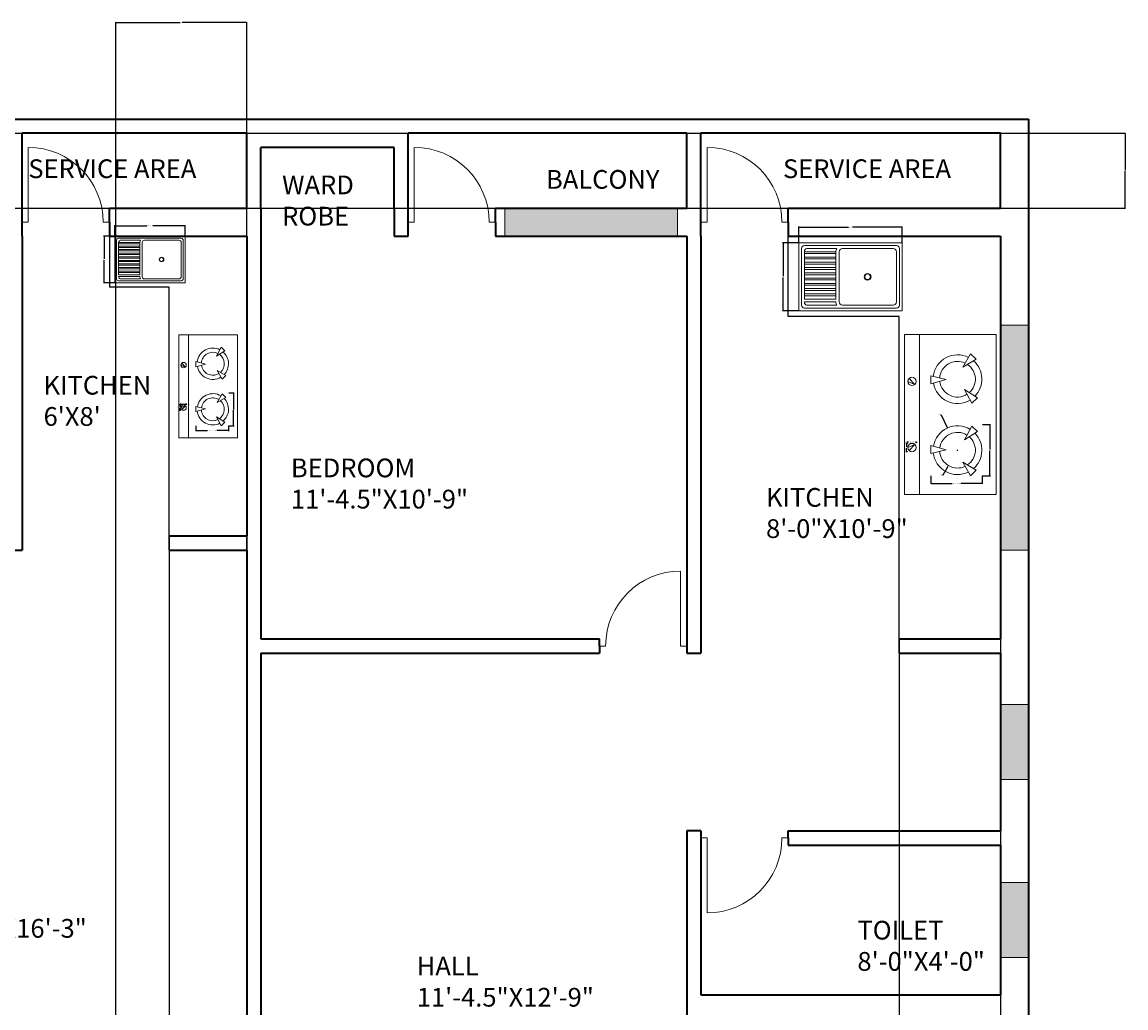
# Model space of a CAD drawing. Units: inches. Extents: x -89 to 565, y -517 to 71.
# Tile 3 of 3: x 211 to 565, y -245 to 71. Entities that reach past the tile are written whole.
import ezdxf

# ---------------------------------------------------------------- set-up
doc = ezdxf.new("R2010")
doc.units = ezdxf.units.IN
doc.header["$MEASUREMENT"] = 0
for name, color, linetype, lineweight in [('A-ANNO-DIMS', 2, 'Continuous', 18), ('A-AREA-IDEN', 7, 'Continuous', 18), ('A-DOOR', 4, 'Continuous', 18), ('A-EQPM', 8, 'Continuous', 18), ('A-FLOR-CASE', 8, 'Continuous', 25), ('A-FLOR-FIXT', 8, 'Continuous', 18), ('A-GLAZ', 3, 'Continuous', 18), ('A-GLAZ-PATT', 9, 'Continuous', 13), ('A-WALL', 7, 'Continuous', 35)]:
    doc.layers.add(name, color=color, linetype=linetype, lineweight=lineweight)
doc.styles.get("Standard").update_dxf_attribs({"font": 'arial.ttf'})
doc.dimstyles.get("Standard").update_dxf_attribs({"dimtxt": 0.18, "dimasz": 0.18, "dimexe": 0.18, "dimexo": 0.0625, "dimgap": 0.09, "dimtad": 0, "dimtih": 1, "dimtoh": 1, "dimdec": 0, "dimzin": 0, "dimdsep": 46, "dimlunit": 3, "dimtxsty": 'Standard', "dimcen": 0.09, "dimadec": 0, "dimazin": 0, "dimtfac": 1, "dimtdec": 0, "dimtofl": 0, "dimtmove": 0, "dimatfit": 3, "dimfxl": 1, "dimtolj": 1, "dimtzin": 0, "dimarcsym": 0})

# ---------------------------------------------------------------- blocks, each defined once
blk = doc.blocks.new('М12 540х820')
for p, q in [((0, 540), (-820, 540)), ((-820, 540), (-820, 0)), ((0, 0), (0, 540)), ((-797.5, 495), (-797.5, 45)), ((-45, 517.5), (-775, 517.5)), ((-775, 468), (-775, 72)), ((-347.5, 495), (-748, 495)), ((-320.5, 468), (-320.5, 72)), ((-301.7, 495), (-64.8, 495)), ((-293.7, 468), (-293.7, 472.5)), ((-293.7, 468), (-45, 468)), ((-293.7, 446.6), (-45, 446.6)), ((-293.7, 419.6), (-293.7, 446.6)), ((-45, 469.5), (-45, 468)), ((-45, 419.6), (-45, 446.6)), ((-22.5, 45), (-22.5, 495)), ((-293.7, 419.6), (-45, 419.6)), ((-293.7, 405), (-45, 405)), ((-293.7, 378), (-293.7, 405)), ((-293.7, 378), (-45, 378)), ((-293.7, 336.4), (-293.7, 363.4)), ((-293.7, 363.4), (-45, 363.4)), ((-45, 378), (-45, 405)), ((-45, 336.4), (-45, 363.4)), ((-293.7, 336.4), (-45, 336.4)), ((-293.7, 294.7), (-293.7, 321.7)), ((-293.7, 321.7), (-45, 321.7)), ((-293.7, 294.7), (-45, 294.7)), ((-293.7, 253.1), (-293.7, 280.1)), ((-293.7, 280.1), (-45, 280.1)), ((-45, 294.7), (-45, 321.7)), ((-45, 253.1), (-45, 280.1)), ((-293.7, 253.1), (-45, 253.1)), ((-293.7, 211.5), (-293.7, 238.5)), ((-293.7, 238.5), (-45, 238.5)), ((-293.7, 211.5), (-45, 211.5)), ((-293.7, 169.9), (-293.7, 196.9)), ((-293.7, 196.9), (-45, 196.9)), ((-45, 211.5), (-45, 238.5)), ((-45, 169.9), (-45, 196.9)), ((-293.7, 169.9), (-45, 169.9)), ((-293.7, 128.2), (-293.7, 155.2)), ((-293.7, 155.2), (-45, 155.2)), ((-293.7, 128.2), (-45, 128.2)), ((-293.7, 113.6), (-45, 113.6)), ((-293.7, 86.6), (-293.7, 113.6)), ((-45, 128.2), (-45, 155.2)), ((-45, 86.6), (-45, 113.6)), ((-820, 0), (0, 0)), ((-775, 22.5), (-45, 22.5)), ((-748, 45), (-347.5, 45)), ((-301.7, 45), (-64.8, 45)), ((-293.7, 86.6), (-45, 86.6)), ((-293.7, 72), (-45, 72)), ((-45, 70.5), (-45, 72))]:
    blk.add_line(p, q)
at = {"ltscale": 0.06}
for p, q in [((-820, 0), (-820, 540)), ((-820, 540), (0, 540)), ((0, 540), (0, 536.9)), ((0, 536.9), (0, 0)), ((-293.7, 446.6), (-45, 446.6)), ((-293.7, 405), (-293.7, 446.6)), ((-45, 446.6), (-45, 419.6)), ((-293.7, 363.4), (-293.7, 405)), ((-293.7, 321.7), (-293.7, 363.4)), ((-45, 419.6), (-45, 378)), ((-45, 378), (-45, 336.4)), ((-293.7, 280.1), (-293.7, 321.7)), ((-293.7, 238.5), (-293.7, 280.1)), ((-45, 336.4), (-45, 294.7)), ((-45, 294.7), (-45, 253.1)), ((-293.7, 196.9), (-293.7, 238.5)), ((-293.7, 155.2), (-293.7, 196.9)), ((-45, 253.1), (-45, 211.5)), ((-45, 211.5), (-45, 169.9)), ((-293.7, 113.6), (-293.7, 155.2)), ((-293.7, 72), (-293.7, 113.6)), ((-45, 169.9), (-45, 128.2)), ((-45, 128.2), (-45, 86.6)), ((0, 0), (-820, 0)), ((-45, 72), (-293.7, 72)), ((-45, 86.6), (-45, 72))]:
    blk.add_line(p, q, dxfattribs=at)
at = {"extrusion": (0, 0, -1)}
for centre, major_axis, start_param, end_param in [((-775, 495), (-15.9, 15.9), -0.785398, 0.785398), ((-775, 495), (-15.9, 15.9), -0.785398, 0.785398), ((-748, 468), (-19.1, -19.1), 0.785398, 2.356194), ((-748, 468), (-19.1, -19.1), 0.785398, 2.356194), ((-347.5, 468), (-19.1, 19.1), 0.785398, 2.356194), ((-347.5, 468), (-19.1, 19.1), 0.785398, 2.356194), ((-343.2, 468), (-35, 35), 1.779263, 2.356194), ((-343.2, 468), (-35, 35), 1.779263, 2.356192), ((-343.2, 468), (-35, 35), 2.356192, 2.356194), ((-72.3, 468.8), (-19.3, 19.3), 1.0328, 2.38382), ((-72.3, 468.8), (-19.3, 19.3), 1.0328, 1.064673), ((-72.3, 468.8), (-19.3, 19.3), 1.064673, 2.328569), ((-45, 495), (-15.9, -15.9), 2.356194, 3.926991), ((-45, 495), (-15.9, -15.9), 2.356194, 3.926991), ((-72.3, 468.8), (-19.3, 19.3), 2.328569, 2.38382), ((-545.5, 270), (-19.1, -19.1), 3.926991, 10.210176), ((-545.5, 270), (-19.1, -19.1), 3.926991, 10.210176), ((-545.5, 270), (-15.9, -15.9), 3.926991, 10.210176), ((-545.5, 270), (-15.9, -15.9), 3.926991, 10.210176), ((-775, 45), (-15.9, -15.9), 5.497787, 7.068583), ((-775, 45), (-15.9, -15.9), 5.497787, 7.068583), ((-748, 72), (-19.1, 19.1), 3.926991, 5.497787), ((-748, 72), (-19.1, 19.1), 3.926991, 5.497787), ((-347.5, 72), (-19.1, -19.1), 3.926991, 5.497787), ((-347.5, 72), (-19.1, -19.1), 3.926991, 5.497787), ((-343.2, 72), (-35, -35), 3.926991, 4.503922), ((-343.2, 72), (-35, -35), 3.926991, 4.503922), ((-72.3, 71.2), (-19.3, -19.3), 3.899365, 5.250385), ((-72.3, 71.2), (-19.3, -19.3), 5.218512, 5.250385), ((-72.3, 71.2), (-19.3, -19.3), 3.954617, 5.218512), ((-72.3, 71.2), (-19.3, -19.3), 3.899365, 3.954617), ((-45, 45), (-15.9, 15.9), 2.356194, 3.926991), ((-45, 45), (-15.9, 15.9), 2.356194, 3.926991)]:
    blk.add_ellipse(centre, major_axis=major_axis, ratio=1, start_param=start_param, end_param=end_param, dxfattribs=at)
blk = doc.blocks.new('DOOR-SWING-24IN')
for p, q in [((0, 0), (0, 24)), ((-24, 0), (-26, 0)), ((2, 0), (0, 0))]:
    blk.add_line(p, q)
blk.add_arc((0, 0), 24, 90, 180)
blk = doc.blocks.new('COOKTOP-BURNER-LARGE')
for p, q in [((2.2, 3.33), (4.59, 7.69)), ((4.59, 7.69), (6.45, 5.97)), ((6.45, 5.97), (2.2, 3.33)), ((-8.51, -1.06), (-8.51, 1.48)), ((-8.51, 1.48), (-3.69, 0.15)), ((-3.69, 0.15), (-8.51, -1.06)), ((4.18, -8.17), (1.75, -3.8)), ((1.75, -3.8), (5.99, -6.39)), ((5.99, -6.39), (4.18, -8.17))]:
    blk.add_line(p, q)
for radius, start, end in [(7.81, 58.853, 170.7562), (5.72, 57.9778, 173.02), (5.72, 304.5561, 48.8027), (7.81, 311.2225, 44.1627), (7.81, 186.4005, 296.769), (5.72, 183.5753, 295.9207)]:
    blk.add_arc((0, 0), radius, start, end)
blk = doc.blocks.new('COOKTOP-KNOB-LARGE')
at = {"ltscale": 20}
for p, q in [((-1.35, 0), (0.95, 0.96)), ((0.95, 0.96), (-0.95, -0.96))]:
    blk.add_line(p, q, dxfattribs=at)
blk.add_circle((0, 0), 1.35, dxfattribs=at)
blk = doc.blocks.new('COOKTOP-BURNER-COMPACT')
for p, q in [((1.41, 2.14), (2.95, 4.94)), ((4.14, 3.83), (1.41, 2.14)), ((2.95, 4.94), (4.14, 3.83)), ((-5.47, -0.68), (-5.47, 0.95)), ((-5.47, 0.95), (-2.37, 0.1)), ((-2.37, 0.1), (-5.47, -0.68)), ((2.69, -5.25), (1.13, -2.44)), ((1.13, -2.44), (3.85, -4.11)), ((3.85, -4.11), (2.69, -5.25))]:
    blk.add_line(p, q)
for radius, start, end in [(5.02, 58.853, 170.7562), (3.68, 57.9778, 173.02), (3.68, 304.5561, 48.8027), (5.02, 311.2225, 44.1627), (5.02, 186.4005, 296.769), (3.68, 183.5753, 295.9207)]:
    blk.add_arc((0, 0), radius, start, end)
blk = doc.blocks.new('COOKTOP-KNOB-COMPACT')
at = {"ltscale": 20}
for p, q in [((-0.87, 0), (0.61, 0.61)), ((0.61, 0.61), (-0.61, -0.61))]:
    blk.add_line(p, q, dxfattribs=at)
blk.add_circle((0, 0), 0.866, dxfattribs=at)
blk = doc.blocks.new('*D14')
at = {"layer": 'A-ANNO-DIMS', "color": 0, "lineweight": -2, "transparency": 16777216}
for p, q in [((240.77, 1.98), (240.77, 5.48)), ((240.95, 5.3), (251.12, 5.3)), ((263.17, 5.3), (252.99, 5.3)), ((263.35, 1.98), (263.35, 5.48))]:
    blk.add_line(p, q, dxfattribs=at)
at = {"layer": 'A-ANNO-DIMS', "color": 0, "transparency": 16777216}
for points in [[(240.95, 5.33), (240.95, 5.27), (240.77, 5.3)], [(263.17, 5.33), (263.17, 5.27), (263.35, 5.3)]]:
    blk.add_solid(points, dxfattribs=at)
at = {"layer": 'Defpoints', "color": 0, "transparency": 16777216}
for p in [(240.77, 5.3), (240.77, 1.91), (263.35, 1.91)]:
    blk.add_point(p, dxfattribs=at)
at = {"layer": 'A-ANNO-DIMS', "color": 0, "transparency": 16777216, "insert": (252.06, 5.3), "char_height": 0.18, "attachment_point": 5}
blk.add_mtext('\\A1;SINK 1\'-10 1/2"', dxfattribs=at)
blk = doc.blocks.new('*D15')
at = {"layer": 'A-ANNO-DIMS', "color": 0, "lineweight": -2, "transparency": 16777216}
for p, q in [((240.71, 1.91), (237.2, 1.91)), ((237.38, 1.73), (237.38, -5.34)), ((237.38, -12.77), (237.38, -5.7)), ((240.71, -12.95), (237.2, -12.95))]:
    blk.add_line(p, q, dxfattribs=at)
at = {"layer": 'A-ANNO-DIMS', "color": 0, "transparency": 16777216}
for points in [[(237.35, 1.73), (237.41, 1.73), (237.38, 1.91)], [(237.35, -12.77), (237.41, -12.77), (237.38, -12.95)]]:
    blk.add_solid(points, dxfattribs=at)
at = {"layer": 'Defpoints', "color": 0, "transparency": 16777216}
for p in [(240.77, 1.91), (237.38, -12.95), (240.77, -12.95)]:
    blk.add_point(p, dxfattribs=at)
at = {"layer": 'A-ANNO-DIMS', "color": 0, "transparency": 16777216, "insert": (237.38, -5.52), "char_height": 0.18, "attachment_point": 5}
blk.add_mtext('\\A1;1\'-3"', dxfattribs=at)
blk = doc.blocks.new('*D16')
at = {"layer": 'A-ANNO-DIMS', "color": 0, "lineweight": -2, "transparency": 16777216}
for p, q in [((459.97, -0.08), (459.97, 5.01)), ((460.15, 4.83), (475.9, 4.83)), ((492.96, 4.83), (477.21, 4.83)), ((493.14, -0.08), (493.14, 5.01))]:
    blk.add_line(p, q, dxfattribs=at)
at = {"layer": 'A-ANNO-DIMS', "color": 0, "transparency": 16777216}
for points in [[(460.15, 4.86), (460.15, 4.8), (459.97, 4.83)], [(492.96, 4.86), (492.96, 4.8), (493.14, 4.83)]]:
    blk.add_solid(points, dxfattribs=at)
at = {"layer": 'Defpoints', "color": 0, "transparency": 16777216}
for p in [(459.97, 4.83), (459.97, -0.14), (493.14, -0.14)]:
    blk.add_point(p, dxfattribs=at)
at = {"layer": 'A-ANNO-DIMS', "color": 0, "transparency": 16777216, "insert": (476.56, 4.83), "char_height": 0.18, "attachment_point": 5}
blk.add_mtext('\\A1;SINK 2\'-9"', dxfattribs=at)
blk = doc.blocks.new('*D17')
at = {"layer": 'A-ANNO-DIMS', "color": 0, "lineweight": -2, "transparency": 16777216}
for p, q in [((459.9, -0.14), (454.81, -0.14)), ((454.99, -0.32), (454.99, -10.89)), ((454.99, -21.81), (454.99, -11.25)), ((459.9, -21.99), (454.81, -21.99))]:
    blk.add_line(p, q, dxfattribs=at)
at = {"layer": 'A-ANNO-DIMS', "color": 0, "transparency": 16777216}
for points in [[(454.96, -0.32), (455.02, -0.32), (454.99, -0.14)], [(454.96, -21.81), (455.02, -21.81), (454.99, -21.99)]]:
    blk.add_solid(points, dxfattribs=at)
at = {"layer": 'Defpoints', "color": 0, "transparency": 16777216}
for p in [(459.97, -0.14), (454.99, -21.99), (459.97, -21.99)]:
    blk.add_point(p, dxfattribs=at)
at = {"layer": 'A-ANNO-DIMS', "color": 0, "transparency": 16777216, "insert": (454.99, -11.07), "char_height": 0.18, "attachment_point": 5}
blk.add_mtext('\\A1;1\'-10"', dxfattribs=at)
blk = doc.blocks.new('*D18')
at = {"layer": 'A-ANNO-DIMS', "color": 0, "lineweight": -2, "transparency": 16777216}
for p, q in [((502.34, -74.83), (502.34, -77.41)), ((502.52, -77.23), (509.13, -77.23)), ((518.56, -77.23), (511.95, -77.23)), ((518.74, -74.83), (518.74, -77.41))]:
    blk.add_line(p, q, dxfattribs=at)
at = {"layer": 'A-ANNO-DIMS', "color": 0, "transparency": 16777216}
for points in [[(502.52, -77.2), (502.52, -77.26), (502.34, -77.23)], [(518.56, -77.2), (518.56, -77.26), (518.74, -77.23)]]:
    blk.add_solid(points, dxfattribs=at)
at = {"layer": 'Defpoints', "color": 0, "transparency": 16777216}
for p in [(502.34, -74.77), (518.74, -74.77), (518.74, -77.23)]:
    blk.add_point(p, dxfattribs=at)
at = {"layer": 'A-ANNO-DIMS', "color": 0, "transparency": 16777216, "insert": (510.54, -77.23), "char_height": 0.18, "attachment_point": 5}
blk.add_mtext('\\A1;BURNER 1\'-4 1/2" TYP.', dxfattribs=at)
blk = doc.blocks.new('*D19')
at = {"layer": 'A-ANNO-DIMS', "color": 0, "lineweight": -2, "transparency": 16777216}
for p, q in [((518.81, -58.42), (521.38, -58.42)), ((521.2, -58.6), (521.2, -66.41)), ((521.2, -74.59), (521.2, -66.78)), ((518.81, -74.77), (521.38, -74.77))]:
    blk.add_line(p, q, dxfattribs=at)
at = {"layer": 'A-ANNO-DIMS', "color": 0, "transparency": 16777216}
for points in [[(521.17, -58.6), (521.23, -58.6), (521.2, -58.42)], [(521.17, -74.59), (521.23, -74.59), (521.2, -74.77)]]:
    blk.add_solid(points, dxfattribs=at)
at = {"layer": 'Defpoints', "color": 0, "transparency": 16777216}
for p in [(518.74, -58.42), (521.2, -58.42), (518.74, -74.77)]:
    blk.add_point(p, dxfattribs=at)
at = {"layer": 'A-ANNO-DIMS', "color": 0, "transparency": 16777216, "insert": (521.2, -66.6), "char_height": 0.18, "attachment_point": 5}
blk.add_mtext('\\A1;1\'-4 1/2" TYP.', dxfattribs=at)
blk = doc.blocks.new('*D20')
at = {"layer": 'A-ANNO-DIMS', "color": 0, "lineweight": -2, "transparency": 16777216}
for p, q in [((494.74, -64.01), (494.56, -64.01)), ((494.92, -64.35), (494.92, -63.83)), ((497.61, -64.35), (497.61, -63.83)), ((497.79, -64.01), (497.97, -64.01))]:
    blk.add_line(p, q, dxfattribs=at)
at = {"layer": 'A-ANNO-DIMS', "color": 0, "transparency": 16777216}
for points in [[(494.74, -63.98), (494.74, -64.04), (494.92, -64.01)], [(497.79, -63.98), (497.79, -64.04), (497.61, -64.01)]]:
    blk.add_solid(points, dxfattribs=at)
at = {"layer": 'Defpoints', "color": 0, "transparency": 16777216}
for p in [(494.92, -64.41), (497.61, -64.01), (497.61, -64.41)]:
    blk.add_point(p, dxfattribs=at)
at = {"layer": 'A-ANNO-DIMS', "color": 0, "transparency": 16777216, "insert": (496.26, -64.01), "char_height": 0.18, "attachment_point": 5}
blk.add_mtext('\\A1;KNOB 0\'-2 1/2" TYP.', dxfattribs=at)
blk = doc.blocks.new('*D21')
at = {"layer": 'A-ANNO-DIMS', "color": 0, "lineweight": -2, "transparency": 16777216}
for p, q in [((494.85, -64.41), (494.33, -64.41)), ((494.85, -67.11), (494.33, -67.11)), ((494.51, -64.59), (494.51, -65.58)), ((494.51, -66.93), (494.51, -65.94))]:
    blk.add_line(p, q, dxfattribs=at)
at = {"layer": 'A-ANNO-DIMS', "color": 0, "transparency": 16777216}
for points in [[(494.48, -64.59), (494.54, -64.59), (494.51, -64.41)], [(494.48, -66.93), (494.54, -66.93), (494.51, -67.11)]]:
    blk.add_solid(points, dxfattribs=at)
at = {"layer": 'Defpoints', "color": 0, "transparency": 16777216}
for p in [(494.51, -64.41), (494.92, -64.41), (494.92, -67.11)]:
    blk.add_point(p, dxfattribs=at)
at = {"layer": 'A-ANNO-DIMS', "color": 0, "transparency": 16777216, "insert": (494.51, -65.76), "char_height": 0.18, "attachment_point": 5}
blk.add_mtext('\\A1;0\'-2 1/2" TYP.', dxfattribs=at)
blk = doc.blocks.new('*D22')
at = {"layer": 'A-ANNO-DIMS', "color": 0, "lineweight": -2, "transparency": 16777216}
for p, q in [((266.75, -58.82), (266.75, -60.52)), ((277.29, -58.82), (277.29, -60.52)), ((266.93, -60.34), (270.54, -60.34)), ((277.11, -60.34), (273.5, -60.34))]:
    blk.add_line(p, q, dxfattribs=at)
at = {"layer": 'A-ANNO-DIMS', "color": 0, "transparency": 16777216}
for points in [[(266.93, -60.31), (266.93, -60.37), (266.75, -60.34)], [(277.11, -60.31), (277.11, -60.37), (277.29, -60.34)]]:
    blk.add_solid(points, dxfattribs=at)
at = {"layer": 'Defpoints', "color": 0, "transparency": 16777216}
for p in [(266.75, -58.76), (277.29, -58.76), (277.29, -60.34)]:
    blk.add_point(p, dxfattribs=at)
at = {"layer": 'A-ANNO-DIMS', "color": 0, "transparency": 16777216, "insert": (272.02, -60.34), "char_height": 0.18, "attachment_point": 5}
blk.add_mtext('\\A1;BURNER 0\'-10 1/2" TYP.', dxfattribs=at)
blk = doc.blocks.new('*D23')
at = {"layer": 'A-ANNO-DIMS', "color": 0, "lineweight": -2, "transparency": 16777216}
for p, q in [((277.35, -48.26), (279.05, -48.26)), ((278.87, -48.44), (278.87, -53.33)), ((278.87, -58.58), (278.87, -53.69)), ((277.35, -58.76), (279.05, -58.76))]:
    blk.add_line(p, q, dxfattribs=at)
at = {"layer": 'A-ANNO-DIMS', "color": 0, "transparency": 16777216}
for points in [[(278.84, -48.44), (278.9, -48.44), (278.87, -48.26)], [(278.84, -58.58), (278.9, -58.58), (278.87, -58.76)]]:
    blk.add_solid(points, dxfattribs=at)
at = {"layer": 'Defpoints', "color": 0, "transparency": 16777216}
for p in [(277.29, -48.26), (278.87, -48.26), (277.29, -58.76)]:
    blk.add_point(p, dxfattribs=at)
at = {"layer": 'A-ANNO-DIMS', "color": 0, "transparency": 16777216, "insert": (278.87, -53.51), "char_height": 0.18, "attachment_point": 5}
blk.add_mtext('\\A1;0\'-10 1/2" TYP.', dxfattribs=at)
blk = doc.blocks.new('*D24')
at = {"layer": 'A-ANNO-DIMS', "color": 0, "lineweight": -2, "transparency": 16777216}
for p, q in [((261.98, -52.04), (261.98, -51.67)), ((262.16, -51.85), (263.53, -51.85)), ((263.71, -52.04), (263.71, -51.67)), ((263.71, -51.85), (263.89, -51.85))]:
    blk.add_line(p, q, dxfattribs=at)
at = {"layer": 'A-ANNO-DIMS', "color": 0, "transparency": 16777216}
for points in [[(262.16, -51.82), (262.16, -51.88), (261.98, -51.85)], [(263.53, -51.82), (263.53, -51.88), (263.71, -51.85)]]:
    blk.add_solid(points, dxfattribs=at)
at = {"layer": 'Defpoints', "color": 0, "transparency": 16777216}
for p in [(261.98, -52.11), (263.71, -51.85), (263.71, -52.11)]:
    blk.add_point(p, dxfattribs=at)
at = {"layer": 'A-ANNO-DIMS', "color": 0, "transparency": 16777216, "insert": (265.13, -51.85), "char_height": 0.18, "attachment_point": 5}
blk.add_mtext('\\A1;KNOB 0\'-1 1/2" TYP.', dxfattribs=at)
blk = doc.blocks.new('*D25')
at = {"layer": 'A-ANNO-DIMS', "color": 0, "lineweight": -2, "transparency": 16777216}
for p, q in [((261.92, -52.11), (261.54, -52.11)), ((261.72, -52.29), (261.72, -52.79)), ((261.92, -53.84), (261.54, -53.84)), ((261.72, -53.66), (261.72, -53.15))]:
    blk.add_line(p, q, dxfattribs=at)
at = {"layer": 'A-ANNO-DIMS', "color": 0, "transparency": 16777216}
for points in [[(261.69, -52.29), (261.75, -52.29), (261.72, -52.11)], [(261.69, -53.66), (261.75, -53.66), (261.72, -53.84)]]:
    blk.add_solid(points, dxfattribs=at)
at = {"layer": 'Defpoints', "color": 0, "transparency": 16777216}
for p in [(261.72, -52.11), (261.98, -52.11), (261.98, -53.84)]:
    blk.add_point(p, dxfattribs=at)
at = {"layer": 'A-ANNO-DIMS', "color": 0, "transparency": 16777216, "insert": (261.72, -52.97), "char_height": 0.18, "attachment_point": 5}
blk.add_mtext('\\A1;0\'-1 1/2" TYP.', dxfattribs=at)
blk = doc.blocks.new('*D26')
at = {"layer": 'A-ANNO-DIMS', "color": 0, "lineweight": -2, "transparency": 16777216}
for p, q in [((241.09, -319.02), (241.09, 70.54)), ((241.27, 70.36), (261.76, 70.36)), ((282.91, 70.36), (262.42, 70.36)), ((283.09, -319.02), (283.09, 70.54))]:
    blk.add_line(p, q, dxfattribs=at)
at = {"layer": 'A-ANNO-DIMS', "color": 0, "transparency": 16777216}
for points in [[(241.27, 70.39), (241.27, 70.33), (241.09, 70.36)], [(282.91, 70.39), (282.91, 70.33), (283.09, 70.36)]]:
    blk.add_solid(points, dxfattribs=at)
at = {"layer": 'Defpoints', "color": 0, "transparency": 16777216}
for p in [(283.09, 70.36), (241.09, -319.09), (283.09, -319.09)]:
    blk.add_point(p, dxfattribs=at)
at = {"layer": 'A-ANNO-DIMS', "color": 0, "transparency": 16777216, "insert": (262.09, 70.36), "char_height": 0.18, "attachment_point": 5}
blk.add_mtext('\\A1;3\'-6"', dxfattribs=at)
blk = doc.blocks.new('*D33')
at = {"layer": 'A-ANNO-DIMS', "color": 0, "lineweight": -2, "transparency": 16777216}
for p, q in [((154.16, 34.91), (564.72, 34.91)), ((564.54, 34.73), (564.54, 23.1)), ((564.54, 11.09), (564.54, 22.73)), ((154.16, 10.91), (564.72, 10.91))]:
    blk.add_line(p, q, dxfattribs=at)
at = {"layer": 'A-ANNO-DIMS', "color": 0, "transparency": 16777216}
for points in [[(564.51, 34.73), (564.57, 34.73), (564.54, 34.91)], [(564.51, 11.09), (564.57, 11.09), (564.54, 10.91)]]:
    blk.add_solid(points, dxfattribs=at)
at = {"layer": 'Defpoints', "color": 0, "transparency": 16777216}
for p in [(154.09, 34.91), (564.54, 34.91), (154.09, 10.91)]:
    blk.add_point(p, dxfattribs=at)
at = {"layer": 'A-ANNO-DIMS', "color": 0, "transparency": 16777216, "insert": (564.54, 22.91), "char_height": 0.18, "attachment_point": 5}
blk.add_mtext('\\A1;2\'-0"', dxfattribs=at)
blk = doc.blocks.new('*D34')
at = {"layer": 'A-ANNO-DIMS', "color": 0, "lineweight": -2, "transparency": 16777216}
for p, q in [((258.18, -94.15), (258.18, -498.72)), ((283.09, -94.15), (283.09, -498.72)), ((258.36, -498.54), (270.31, -498.54)), ((282.91, -498.54), (270.97, -498.54))]:
    blk.add_line(p, q, dxfattribs=at)
at = {"layer": 'A-ANNO-DIMS', "color": 0, "transparency": 16777216}
for points in [[(258.36, -498.51), (258.36, -498.57), (258.18, -498.54)], [(282.91, -498.51), (282.91, -498.57), (283.09, -498.54)]]:
    blk.add_solid(points, dxfattribs=at)
at = {"layer": 'Defpoints', "color": 0, "transparency": 16777216}
for p in [(258.18, -94.09), (283.09, -94.09), (283.09, -498.54)]:
    blk.add_point(p, dxfattribs=at)
at = {"layer": 'A-ANNO-DIMS', "color": 0, "transparency": 16777216, "insert": (270.64, -498.54), "char_height": 0.18, "attachment_point": 5}
blk.add_mtext('\\A1;2\'-1"', dxfattribs=at)
blk = doc.blocks.new('*D35')
at = {"layer": 'A-ANNO-DIMS', "color": 0, "lineweight": -2, "transparency": 16777216}
for p, q in [((492.2, -127.15), (492.2, -498.72)), ((524.59, -127.15), (524.59, -498.72)), ((492.38, -498.54), (507.86, -498.54)), ((524.41, -498.54), (508.94, -498.54))]:
    blk.add_line(p, q, dxfattribs=at)
at = {"layer": 'A-ANNO-DIMS', "color": 0, "transparency": 16777216}
for points in [[(492.38, -498.51), (492.38, -498.57), (492.2, -498.54)], [(524.41, -498.51), (524.41, -498.57), (524.59, -498.54)]]:
    blk.add_solid(points, dxfattribs=at)
at = {"layer": 'Defpoints', "color": 0, "transparency": 16777216}
for p in [(492.2, -127.09), (524.59, -127.09), (524.59, -498.54)]:
    blk.add_point(p, dxfattribs=at)
at = {"layer": 'A-ANNO-DIMS', "color": 0, "transparency": 16777216, "insert": (508.4, -498.54), "char_height": 0.18, "attachment_point": 5}
blk.add_mtext('\\A1;2\'-8 1/2"', dxfattribs=at)
blk = doc.blocks.new('*D36')
at = {"layer": 'A-ANNO-DIMS', "color": 0, "lineweight": -2, "transparency": 16777216}
for p, q in [((505.42, -55.26), (505.6, -55.26)), ((505.6, -55.26), (507.5, -59.35)), ((510.76, -66.61), (510.94, -66.61)), ((510.85, -66.7), (510.85, -66.52))]:
    blk.add_line(p, q, dxfattribs=at)
at = {"layer": 'A-ANNO-DIMS', "color": 0, "transparency": 16777216}
blk.add_solid([(507.52, -59.34), (507.47, -59.36), (507.57, -59.51)], dxfattribs=at)
at = {"layer": 'Defpoints', "color": 0, "transparency": 16777216}
for p in [(507.57, -59.51), (510.85, -66.61)]:
    blk.add_point(p, dxfattribs=at)
at = {"layer": 'A-ANNO-DIMS', "color": 0, "transparency": 16777216, "insert": (505.01, -55.26), "char_height": 0.18, "attachment_point": 5}
blk.add_mtext('\\A1;R0\'-8"', dxfattribs=at)
blk = doc.blocks.new('*D37')
at = {"layer": 'A-ANNO-DIMS', "color": 0, "lineweight": -2, "transparency": 16777216}
for p, q in [((510.76, -66.61), (510.94, -66.61)), ((510.85, -66.7), (510.85, -66.52)), ((506.24, -74.52), (507.88, -71.71)), ((506.06, -74.52), (506.24, -74.52))]:
    blk.add_line(p, q, dxfattribs=at)
at = {"layer": 'A-ANNO-DIMS', "color": 0, "transparency": 16777216}
blk.add_solid([(507.85, -71.69), (507.9, -71.72), (507.97, -71.55)], dxfattribs=at)
at = {"layer": 'Defpoints', "color": 0, "transparency": 16777216}
for p in [(510.85, -66.61), (507.97, -71.55)]:
    blk.add_point(p, dxfattribs=at)
at = {"layer": 'A-ANNO-DIMS', "color": 0, "transparency": 16777216, "insert": (505.44, -74.52), "char_height": 0.18, "attachment_point": 5}
blk.add_mtext('\\A1;R0\'-5 1/2"', dxfattribs=at)

msp = doc.modelspace()

# ---------------------------------------------------------------- hatches: boundary and pattern name
at = {"layer": 'A-GLAZ-PATT'}
h = msp.add_hatch(dxfattribs=at)
h.set_pattern_fill('GOST_WOOD', color=256)
h.set_pattern_definition([(90, (0, 0), (6, -4e-16), [10, -2]), (90, (2, -2), (6, -4e-16), [6, -1.5, 3, -1.5]), (90, (4, -5), (6, -4e-16), [10, -2])])
h.paths.add_polyline_path([(46.09, -73.09), (41.59, -73.09), (37.09, -73.09), (37.09, -133.09), (41.59, -133.09), (46.09, -133.09)])
h.paths.add_polyline_path([(46.09, -175.84), (41.59, -175.84), (37.09, -175.84), (37.09, -223.84), (41.59, -223.84), (46.09, -223.84)])
h.paths.add_polyline_path([(46.09, -257.59), (41.59, -257.59), (37.09, -257.59), (37.09, -281.59), (41.59, -281.59), (46.09, -281.59)])
h.paths.add_polyline_path([(140.84, -418.09), (68.84, -418.09), (68.84, -422.59), (68.84, -427.09), (140.84, -427.09), (140.84, -422.59)])
h.paths.add_polyline_path([(501.84, -418.09), (429.84, -418.09), (429.84, -422.59), (429.84, -427.09), (501.84, -427.09), (501.84, -422.59)])
h.paths.add_polyline_path([(533.59, -322.09), (529.09, -322.09), (524.59, -322.09), (524.59, -394.09), (529.09, -394.09), (533.59, -394.09)])
h.paths.add_polyline_path([(533.59, -257.59), (529.09, -257.59), (524.59, -257.59), (524.59, -281.59), (529.09, -281.59), (533.59, -281.59)])
h.paths.add_polyline_path([(533.59, -205.09), (529.09, -205.09), (524.59, -205.09), (524.59, -229.09), (529.09, -229.09), (533.59, -229.09)])
h.paths.add_polyline_path([(533.59, -148.09), (529.09, -148.09), (524.59, -148.09), (524.59, -172.09), (529.09, -172.09), (533.59, -172.09)])
h.paths.add_polyline_path([(533.59, -26.59), (529.09, -26.59), (524.59, -26.59), (524.59, -98.59), (529.09, -98.59), (533.59, -98.59)])
h.paths.add_polyline_path([(421.09, 10.91), (365.78, 10.91), (365.78, 1.91), (421.09, 1.91)])
h.paths.add_polyline_path([(194.59, 10.91), (170.59, 10.91), (170.59, 1.91), (194.59, 1.91)])

# ---------------------------------------------------------------- linework, layer by layer
at = {"layer": 'A-EQPM'}
for p, q in [((264.38, -62.63), (264.38, -29.7)), ((498.65, -80.8), (498.65, -29.53))]:
    msp.add_line(p, q, dxfattribs=at)
for points in [[(280.14, -29.7), (280.14, -62.63), (261.32, -62.63), (261.32, -29.7)], [(523.19, -29.53), (523.19, -80.8), (493.89, -80.8), (493.89, -29.53)]]:
    msp.add_lwpolyline(points, close=True, dxfattribs=at)
at = {"layer": 'A-FLOR-CASE'}
for p, q in [((239.09, 1.91), (239.09, -14.42)), ((456.59, -23.79), (456.59, 1.91)), ((258.18, -14.42), (239.09, -14.42)), ((258.18, -98.59), (258.18, -14.42)), ((492.2, -23.79), (456.59, -23.79)), ((492.2, -131.59), (492.2, -23.79))]:
    msp.add_line(p, q, dxfattribs=at)
at = {"layer": 'A-GLAZ'}
for p, q in [((365.78, 10.91), (365.78, 1.91)), ((421.09, 10.91), (421.09, 1.91)), ((529.09, -26.59), (524.59, -26.59)), ((529.09, -26.59), (533.59, -26.59)), ((529.09, -98.59), (524.59, -98.59)), ((529.09, -98.59), (533.59, -98.59)), ((529.09, -148.09), (524.59, -148.09)), ((529.09, -148.09), (533.59, -148.09)), ((524.59, -160.09), (524.59, -160.09)), ((529.09, -172.09), (524.59, -172.09)), ((529.09, -172.09), (533.59, -172.09)), ((529.09, -205.09), (524.59, -205.09)), ((529.09, -205.09), (533.59, -205.09)), ((529.09, -229.09), (524.59, -229.09)), ((529.09, -229.09), (533.59, -229.09))]:
    msp.add_line(p, q, dxfattribs=at)
at = {"layer": 'A-WALL'}
for p, q in [((206.59, 39.41), (533.59, 39.41)), ((533.59, 39.41), (533.59, 10.91)), ((211.09, 10.91), (211.09, 34.91)), ((283.09, 34.91), (211.09, 34.91)), ((283.09, 10.91), (283.09, 34.91)), ((424.09, 34.91), (334.78, 34.91)), ((334.78, 10.91), (334.78, 34.91)), ((424.09, 10.91), (424.09, 34.91)), ((524.59, 34.91), (428.59, 34.91)), ((428.59, 10.91), (428.59, 34.91)), ((524.59, 10.91), (524.59, 34.91)), ((287.59, 10.91), (287.59, 30.41)), ((330.28, 30.41), (287.59, 30.41)), ((330.28, 10.91), (330.28, 30.41)), ((211.09, 1.91), (211.09, 10.91)), ((239.09, 6.41), (239.09, 10.91)), ((239.09, 10.91), (283.09, 10.91)), ((287.59, 10.91), (287.59, 1.91)), ((330.28, 10.91), (330.28, 1.91)), ((334.78, 1.91), (334.78, 10.91)), ((362.78, 6.41), (362.78, 10.91)), ((362.78, 10.91), (424.09, 10.91)), ((428.59, 1.91), (428.59, 10.91)), ((456.59, 6.41), (456.59, 10.91)), ((456.59, 10.91), (524.59, 10.91)), ((533.59, 10.91), (533.59, -467.59)), ((239.09, 6.41), (239.09, 1.91)), ((362.78, 6.41), (362.78, 1.91)), ((456.59, 6.41), (456.59, 1.91)), ((211.09, 1.91), (211.09, -98.59)), ((239.09, 1.91), (283.09, 1.91)), ((283.09, 1.91), (283.09, -94.09)), ((287.59, 1.91), (287.59, -127.09)), ((330.28, 1.91), (334.78, 1.91)), ((362.78, 1.91), (424.09, 1.91)), ((424.09, 1.91), (424.09, -131.59)), ((428.59, 1.91), (428.59, -131.59)), ((456.59, 1.91), (524.59, 1.91)), ((524.59, 1.91), (524.59, -127.09)), ((258.18, -94.09), (283.09, -94.09)), ((206.59, -98.59), (211.09, -98.59)), ((258.18, -98.59), (283.09, -98.59)), ((283.09, -98.59), (283.09, -298.09)), ((287.59, -127.09), (396.09, -127.09)), ((396.09, -129.34), (396.09, -127.09)), ((492.2, -127.09), (524.59, -127.09)), ((396.09, -129.34), (396.09, -131.59)), ((287.59, -131.59), (396.09, -131.59)), ((287.59, -131.59), (287.59, -298.09)), ((424.09, -131.59), (428.59, -131.59)), ((492.2, -131.59), (524.59, -131.59)), ((524.59, -131.59), (524.59, -188.59)), ((428.59, -188.59), (424.09, -188.59)), ((424.09, -188.59), (424.09, -293.59)), ((428.59, -188.59), (428.59, -241.09)), ((456.59, -188.59), (524.59, -188.59)), ((456.59, -190.84), (456.59, -188.59)), ((456.59, -190.84), (456.59, -193.09)), ((456.59, -193.09), (524.59, -193.09)), ((524.59, -193.09), (524.59, -241.09)), ((428.59, -241.09), (524.59, -241.09))]:
    msp.add_line(p, q, dxfattribs=at)

# ---------------------------------------------------------------- block references
at = {"layer": 'A-DOOR', "extrusion": (0, 0, -1), "zscale": -1}
for p in [(-213.09, 6.41), (-336.78, 6.41), (-430.59, 6.41)]:
    msp.add_blockref('DOOR-SWING-24IN', p, dxfattribs=at)
at = {"layer": 'A-DOOR'}
msp.add_blockref('DOOR-SWING-24IN', (422.09, -129.34), dxfattribs=at)
at = {"layer": 'A-DOOR', "rotation": 180}
msp.add_blockref('DOOR-SWING-24IN', (430.59, -190.84), dxfattribs=at)
at = {"layer": 'A-EQPM', "extrusion": (0, 0, -1), "zscale": -1, "rotation": 180}
for name, p in [('COOKTOP-BURNER-COMPACT', (-272.22, -38.9)), ('COOKTOP-KNOB-COMPACT', (-262.85, -39.36)), ('COOKTOP-BURNER-LARGE', (-510.85, -43.86)), ('COOKTOP-KNOB-LARGE', (-496.26, -44.57))]:
    msp.add_blockref(name, p, dxfattribs=at)
at = {"layer": 'A-EQPM'}
for name, p in [('COOKTOP-BURNER-COMPACT', (272.22, -53.51)), ('COOKTOP-KNOB-COMPACT', (262.85, -52.97)), ('COOKTOP-BURNER-LARGE', (510.85, -66.61)), ('COOKTOP-KNOB-LARGE', (496.26, -65.76))]:
    msp.add_blockref(name, p, dxfattribs=at)
at = {"layer": 'A-FLOR-FIXT', "rotation": 180}
for p, xscale, yscale, zscale in [((240.77, 1.91), 0.0275342750291305, 0.0275342750291305, 0.0275342750291305), ((459.97, -0.14), 0.0404612055524312, 0.0404612055524312, 0.0404612055524312)]:
    msp.add_blockref('М12 540х820', p, dxfattribs=dict(at, xscale=xscale, yscale=yscale, zscale=zscale))

# ---------------------------------------------------------------- texts
at = {"layer": 'A-AREA-IDEN', "char_height": 6, "attachment_point": 1}
for s, insert in [('SERVICE AREA', (213.09, 26.57)), ('SERVICE AREA', (454.92, 26.57)), ('WARD\\PROBE', (294.41, 21.37)), ('BALCONY', (378.98, 23.15)), ("KITCHEN\\P6'X8'", (217.98, -42.8)), ('BEDROOM\\P11\'-4.5"X10\'-9"', (297.24, -69.29)), ('KITCHEN\\P8\'-0"X10\'-9"', (449.49, -78.73)), ('HALL\\P19\'-9"X16\'-3"', (181.9, -206.79)), ('TOILET\\P8\'-0"X4\'-0"', (478.77, -217.38)), ('HALL\\P11\'-4.5"X12\'-9"', (337.57, -228.87))]:
    msp.add_mtext(s, dxfattribs=dict(at, insert=insert))

# ---------------------------------------------------------------- dimensions: what is measured, and where the dimension line sits
at = {"layer": 'A-ANNO-DIMS'}
for base, p1, p2, picture, middle in [((283.09, 70.36), (241.09, -319.09), (283.09, -319.09), '*D26', (262.09, 70.36)), ((283.09, -498.54), (258.18, -94.09), (283.09, -94.09), '*D34', (270.64, -498.54)), ((524.59, -498.54), (492.2, -127.09), (524.59, -127.09), '*D35', (508.4, -498.54))]:
    dim = msp.add_linear_dim(base=base, p1=p1, p2=p2, dimstyle='Standard', override={"dimdec": 1, "dimlfac": 1, "dimrnd": 0, "dimzin": 1, "dimdsep": 46, "dimlunit": 4, "dimfrac": 2}, dxfattribs=at)
    dim.commit()
    dim.dimension.update_dxf_attribs({"geometry": picture, "text_midpoint": middle})
for base, p1, p2, angle, picture, middle in [((564.54, 34.91), (154.09, 10.91), (154.09, 34.91), 90, '*D33', (564.54, 22.91)), ((237.38, -12.95), (240.77, 1.91), (240.77, -12.95), 270, '*D15', (237.38, -5.52)), ((454.9893, -21.9935), (459.966, -0.1445), (459.966, -21.9935), 270, '*D17', (454.9893, -11.069))]:
    dim = msp.add_linear_dim(base=base, p1=p1, p2=p2, angle=angle, dimstyle='Standard', override={"dimdec": 1, "dimlfac": 1, "dimrnd": 0, "dimzin": 1, "dimdsep": 46, "dimlunit": 4, "dimfrac": 2}, dxfattribs=at)
    dim.commit()
    dim.dimension.update_dxf_attribs({"geometry": picture, "text_midpoint": middle})
for base, p1, p2, angle, text, picture, middle in [((240.77, 5.3), (263.35, 1.91), (240.77, 1.91), 180, 'SINK <>', '*D14', (252.06, 5.3)), ((459.97, 4.83), (493.14, -0.14), (459.97, -0.14), 180, 'SINK <>', '*D16', (476.56, 4.83)), ((278.87, -48.26), (277.29, -58.76), (277.29, -48.26), 90, '<> TYP.', '*D23', (278.87, -53.51)), ((261.72, -52.11), (261.98, -53.84), (261.98, -52.11), 90, '<> TYP.', '*D25', (261.72, -52.97)), ((521.2049, -58.4236), (518.7438, -74.7725), (518.7438, -58.4236), 90, '<> TYP.', '*D19', (521.2049, -66.5981)), ((494.51, -64.41), (494.92, -67.11), (494.92, -64.41), 90, '<> TYP.', '*D21', (494.51, -65.76))]:
    dim = msp.add_linear_dim(base=base, p1=p1, p2=p2, angle=angle, text=text, dimstyle='Standard', override={"dimdec": 1, "dimlfac": 1, "dimrnd": 0, "dimzin": 1, "dimdsep": 46, "dimlunit": 4, "dimfrac": 2}, dxfattribs=at)
    dim.commit()
    dim.dimension.update_dxf_attribs({"geometry": picture, "text_midpoint": middle})
for base, p1, p2, text, picture, middle in [((263.71, -51.85), (261.98, -52.11), (263.71, -52.11), 'KNOB <> TYP.', '*D24', (265.13, -51.85)), ((277.29, -60.34), (266.75, -58.76), (277.29, -58.76), 'BURNER <> TYP.', '*D22', (272.02, -60.34)), ((497.61, -64.01), (494.92, -64.41), (497.61, -64.41), 'KNOB <> TYP.', '*D20', (496.26, -64.01)), ((518.74, -77.23), (502.34, -74.77), (518.74, -74.77), 'BURNER <> TYP.', '*D18', (510.54, -77.23))]:
    dim = msp.add_linear_dim(base=base, p1=p1, p2=p2, text=text, dimstyle='Standard', override={"dimdec": 1, "dimlfac": 1, "dimrnd": 0, "dimzin": 1, "dimdsep": 46, "dimlunit": 4, "dimfrac": 2}, dxfattribs=at)
    dim.commit()
    dim.dimension.update_dxf_attribs({"geometry": picture, "text_midpoint": middle})
for mpoint, picture, middle in [((507.57, -59.51), '*D36', (505.01, -55.26)), ((507.97, -71.55), '*D37', (505.44, -74.52))]:
    dim = msp.add_radius_dim(center=(510.85, -66.61), mpoint=mpoint, dimstyle='Standard', override={"dimdec": 1, "dimlfac": 1, "dimrnd": 0, "dimzin": 1, "dimdsep": 46, "dimlunit": 4, "dimfrac": 2}, dxfattribs=at)
    dim.commit()
    dim.dimension.update_dxf_attribs({"geometry": picture, "text_midpoint": middle, "dimtype": 164})

doc.saveas('drawing.dxf')
